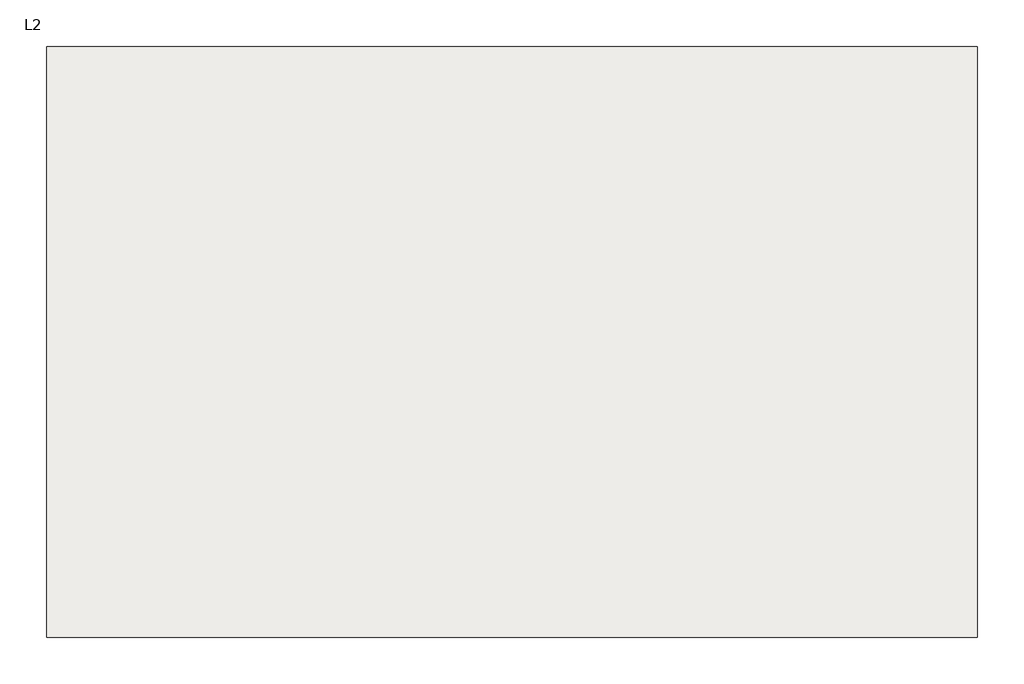
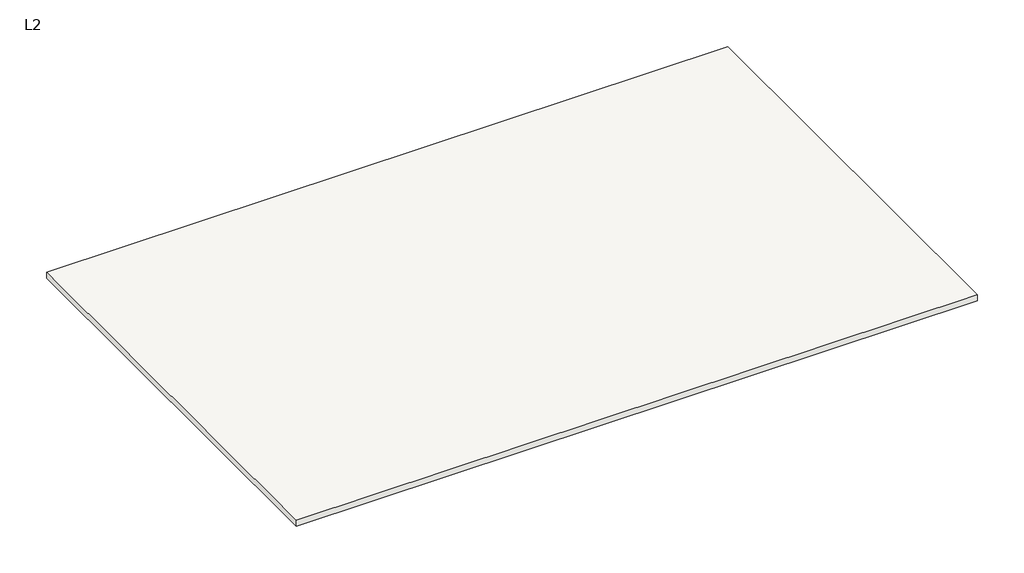
# One storey: 1 slab.
"""IFC4 building model written with IfcOpenShell, lengths in millimetres."""

from ifc_helpers import new_model, si_unit, frame, origin, place, context, project, spatial, polyline, outline, extrude, element, save

model = new_model("IFC4")

# Units and contexts
model_context = context("Model", 3, world=origin())
ifc_project = project(units=[si_unit("LENGTHUNIT", "METRE", prefix="MILLI")], contexts=[model_context])

# Site, building, storey
site = spatial("IfcSite", under=ifc_project)
building = spatial("IfcBuilding", under=site)
storey = spatial("IfcBuildingStorey", under=building, Name="L2", Elevation=3657.6)

# Slab
placement = place(None, origin())
element("IfcSlab", 1, ObjectType="slab 6\"", at=placement, inside=storey, context=model_context, shape_type="SweptSolid", body=[
    extrude(outline(polyline([(10435.3120815, 5448.8278379), (10435.3120815, -4990.5721621), (-5998.4879185, -4990.5721621), (-5998.4879185, 5448.8278379), (10435.3120815, 5448.8278379)])), frame((0.0, 0.0, 3505.2), z_axis=(0.0, 0.0, 1.0), x_axis=(1.0, 0.0, 0.0)), (0.0, 0.0, 1.0), 152.4),
])

save(model, "model.ifc")

# Revit data of these elements
# Type "slab 6\""
#   Description = "Generic Floor (Material By Category), 12\" thick"
#   Assembly Code = "B1010"
#   Type Mark = "G01"
#   Function = 0
#   Layers, outside or top first: 0' - 6" no material (function 1)
# Element 1 (IfcSlab, "slab 6\"")
#   Height Offset From Level = 0' - 0"
#   Phase Created = New Construction
#   Materials on its faces: "Default Floor"
# Materials
#   "Default Floor": colour RGB 128 128 128, transparency 0, Cost = 0
